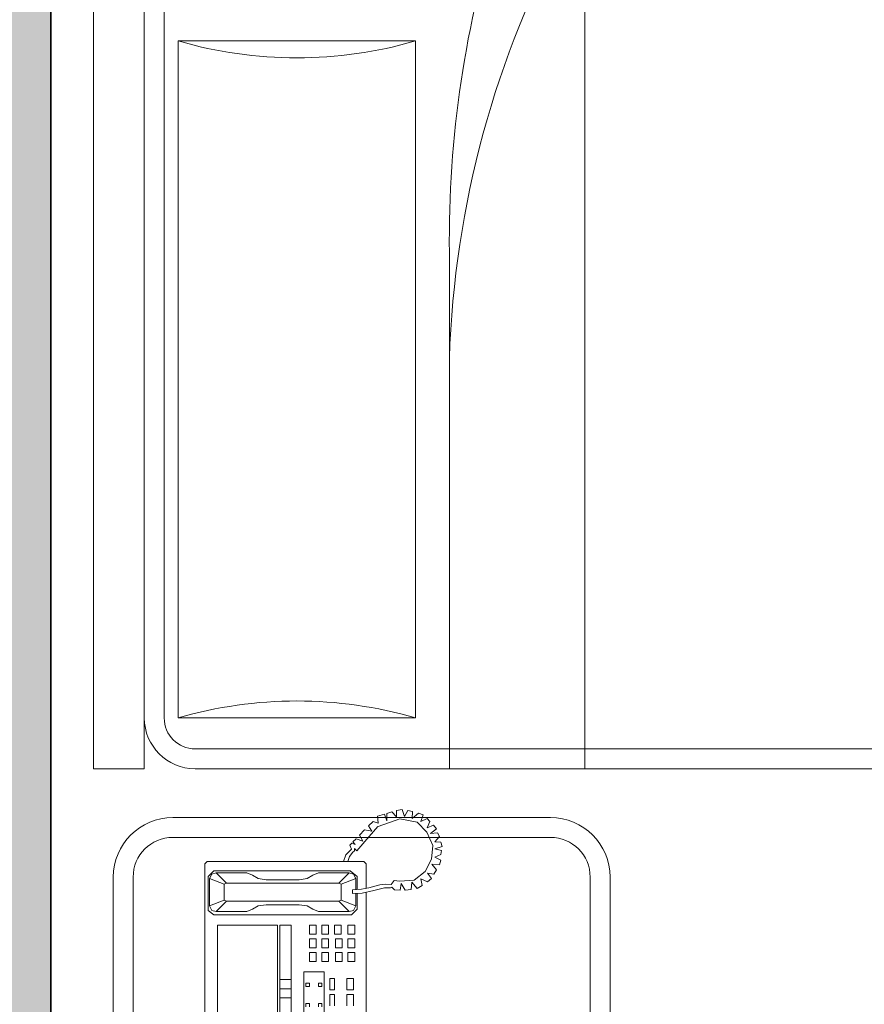
# Model space of a CAD drawing. Units: inches. Extents: x 2701 to 6846, y 811 to 2447.
# Tile 17 of 20: x 2977 to 3008, y 1370 to 1407. Entities that reach past the tile are written whole.
import ezdxf

# ---------------------------------------------------------------- set-up
doc = ezdxf.new("R2010")
doc.units = ezdxf.units.IN
for name, color, linetype, lineweight in [('A-FLOR-PATT', 252, 'Continuous', 13), ('A-FURN', 8, 'Continuous', 13), ('A-WALL', 7, 'Continuous', 35)]:
    doc.layers.add(name, color=color, linetype=linetype, lineweight=lineweight)
doc.layers.add('A-WALL-PATT', color=18, linetype='Continuous', lineweight=13, true_color=0x000000)

# ---------------------------------------------------------------- blocks, each defined once
blk = doc.blocks.new('A$C356F0359')
for p, q in [((0.5488961549126543, 2.000037877005524), (2.049197857799299, 2.000037877005524)), ((0.5488961549126543, 1.948857180890627), (0.5488961549126543, 2.000037877005524)), ((0.4397736946484656, 1.980067907948978), (0.059773694651085, 1.980067907948978)), ((0.4397736946484656, 1.960067907952179), (0.059773694651085, 1.960067907952179)), ((2.049197857799299, 1.948857180890627), (0.5488961549126543, 1.948857180890627)), ((1.998017161684401, 1.928857180893828), (0.6000768510275521, 1.928857180893828)), ((0.4797736946493388, 1.540067907953925), (0.4797736946493388, 1.920067907951306)), ((0.4997736946534133, 1.540067907953925), (0.4997736946534133, 1.920067907951306)), ((0.5488961549126543, 1.897676484783005), (0.5488961549126543, 0.0512185731204227)), ((0.5688961549167288, 1.897676484783005), (0.5688961549167288, 0.0512185731204227)), ((0.2724584284442244, 1.887891571575892), (0.4530524284491549, 1.887891571575892)), ((0.4016174284479348, 1.878747571572603), (0.4061894284459413, 1.88446257157193)), ((0.4061894284459413, 1.88446257157193), (0.44047942844918, 1.88446257157193)), ((0.44047942844918, 1.88446257157193), (0.4461944284485071, 1.878747571572603)), ((0.4530524284491549, 1.887891571575892), (0.4553384284445201, 1.88560557157325)), ((0.4553384284445201, 1.88560557157325), (0.4553384284445201, 1.727871571572904)), ((0.3913304284506012, 1.875318571575917), (0.2770304284495069, 1.875318571575917)), ((0.3913304284506012, 1.814739571571408), (0.3913304284506012, 1.875318571575917)), ((0.4016174284479348, 1.740444571572879), (0.4016174284479348, 1.878747571572603)), ((0.4061894284459413, 1.881033571575244), (0.4050464284446207, 1.876461571577237)), ((0.4050464284446207, 1.876461571577237), (0.4153334284492303, 1.866174571572628)), ((0.4050464284446207, 1.876461571577237), (0.4050464284446207, 1.845600571570685)), ((0.4107614284439478, 1.883319571570609), (0.4061894284459413, 1.881033571575244)), ((0.4107614284439478, 1.883319571570609), (0.4381934284465388, 1.883319571570609)), ((0.4164764284505509, 1.868460571575269), (0.4107614284439478, 1.883319571570609)), ((0.4324784284472117, 1.868460571575269), (0.4381934284465388, 1.883319571570609)), ((0.4439084284458659, 1.876461571577237), (0.4336214284485323, 1.866174571572628)), ((0.4381934284465388, 1.883319571570609), (0.4427654284445453, 1.881033571575244)), ((0.4427654284445453, 1.881033571575244), (0.4439084284458659, 1.876461571577237)), ((0.4439084284458659, 1.876461571577237), (0.4439084284458659, 1.845600571570685)), ((0.4461944284485071, 1.878747571572603), (0.4461944284485071, 1.7415875715742)), ((0.4153334284492303, 1.866174571572628), (0.4164764284505509, 1.868460571575269)), ((0.4153334284492303, 1.814739571571408), (0.4153334284492303, 1.866174571572628)), ((0.4324784284472117, 1.868460571575269), (0.4164764284505509, 1.868460571575269)), ((0.4336214284485323, 1.866174571572628), (0.4324784284472117, 1.868460571575269)), ((0.4336214284485323, 1.814739571571408), (0.4336214284485323, 1.866174571572628)), ((0.4050464284446207, 1.845600571570685), (0.407332428447262, 1.839885571571358)), ((0.4439084284458659, 1.845600571570685), (0.4416224284505006, 1.839885571571358)), ((0.407332428447262, 1.839885571571358), (0.4107614284439478, 1.83417057157203)), ((0.4416224284505006, 1.839885571571358), (0.4381934284465388, 1.83417057157203)), ((0.4107614284439478, 1.83417057157203), (0.4119044284452685, 1.826169571577338)), ((0.4119044284452685, 1.826169571577338), (0.4119044284452685, 1.814739571571408)), ((0.4381934284465388, 1.83417057157203), (0.4370504284452182, 1.826169571577338)), ((0.4370504284452182, 1.826169571577338), (0.4370504284452182, 1.814739571571408)), ((0.2770304284495069, 1.814739571571408), (0.3913304284506012, 1.814739571571408)), ((0.3913304284506012, 1.812453571576043), (0.2816024284475134, 1.812453571576043)), ((0.3181784284461173, 1.812453571576043), (0.3181784284461173, 1.801023571577388)), ((0.3273224284494063, 1.812453571576043), (0.3273224284494063, 1.801023571577388)), ((0.3364664284454193, 1.812453571576043), (0.3364664284454193, 1.801023571577388)), ((0.3913304284506012, 1.801023571577388), (0.3913304284506012, 1.812453571576043)), ((0.4119044284452685, 1.79302257157542), (0.4119044284452685, 1.814739571571408)), ((0.4153334284492303, 1.814739571571408), (0.4153334284492303, 1.753017571572854)), ((0.4336214284485323, 1.814739571571408), (0.4336214284485323, 1.753017571572854)), ((0.4370504284452182, 1.79302257157542), (0.4370504284452182, 1.814739571571408)), ((0.2816024284475134, 1.801023571577388), (0.3913304284506012, 1.801023571577388)), ((0.3444674284473876, 1.788450571577413), (0.2770304284495069, 1.788450571577413)), ((0.3124634284467902, 1.786164571574772), (0.3090344284501043, 1.786164571574772)), ((0.3124634284467902, 1.78273557157081), (0.3124634284467902, 1.786164571574772)), ((0.3330374284487334, 1.786164571574772), (0.3296084284447716, 1.786164571574772)), ((0.3296084284447716, 1.786164571574772), (0.3296084284447716, 1.78273557157081)), ((0.3330374284487334, 1.78273557157081), (0.3330374284487334, 1.786164571574772)), ((0.3444674284473876, 1.76787657157547), (0.3444674284473876, 1.788450571577413)), ((0.4107614284439478, 1.785021571573452), (0.4119044284452685, 1.79302257157542)), ((0.4381934284465388, 1.785021571573452), (0.4370504284452182, 1.79302257157542)), ((0.3090344284501043, 1.78273557157081), (0.3124634284467902, 1.78273557157081)), ((0.3296084284447716, 1.78273557157081), (0.3330374284487334, 1.78273557157081)), ((0.3547544284447213, 1.775877571577439), (0.3547544284447213, 1.78273557157081)), ((0.3547544284447213, 1.78273557157081), (0.3638984284480102, 1.78273557157081)), ((0.3638984284480102, 1.775877571577439), (0.3547544284447213, 1.775877571577439)), ((0.3638984284480102, 1.78273557157081), (0.3638984284480102, 1.775877571577439)), ((0.3684704284460167, 1.78273557157081), (0.3776144284493057, 1.78273557157081)), ((0.3684704284460167, 1.775877571577439), (0.3684704284460167, 1.78273557157081)), ((0.3776144284493057, 1.775877571577439), (0.3684704284460167, 1.775877571577439)), ((0.3776144284493057, 1.78273557157081), (0.3776144284493057, 1.775877571577439)), ((0.3821864284473122, 1.775877571577439), (0.3821864284473122, 1.78273557157081)), ((0.3821864284473122, 1.78273557157081), (0.3913304284506012, 1.78273557157081)), ((0.3913304284506012, 1.775877571577439), (0.3821864284473122, 1.775877571577439)), ((0.3913304284506012, 1.78273557157081), (0.3913304284506012, 1.775877571577439)), ((0.4050464284446207, 1.773591571574797), (0.407332428447262, 1.779306571574124)), ((0.407332428447262, 1.779306571574124), (0.4107614284439478, 1.785021571573452)), ((0.4416224284505006, 1.779306571574124), (0.4381934284465388, 1.785021571573452)), ((0.4439084284458659, 1.773591571574797), (0.4416224284505006, 1.779306571574124)), ((0.2770304284495069, 1.76787657157547), (0.3444674284473876, 1.76787657157547)), ((0.3124634284467902, 1.773591571574797), (0.3090344284501043, 1.773591571574797)), ((0.3090344284501043, 1.770162571570836), (0.3124634284467902, 1.770162571570836)), ((0.3124634284467902, 1.770162571570836), (0.3124634284467902, 1.773591571574797)), ((0.3330374284487334, 1.773591571574797), (0.3296084284447716, 1.773591571574797)), ((0.3296084284447716, 1.773591571574797), (0.3296084284447716, 1.770162571570836)), ((0.3296084284447716, 1.770162571570836), (0.3330374284487334, 1.770162571570836)), ((0.3330374284487334, 1.770162571570836), (0.3330374284487334, 1.773591571574797)), ((0.3547544284447213, 1.763304571577464), (0.3547544284447213, 1.770162571570836)), ((0.3547544284447213, 1.770162571570836), (0.3638984284480102, 1.770162571570836)), ((0.3638984284480102, 1.770162571570836), (0.3638984284480102, 1.763304571577464)), ((0.3684704284460167, 1.763304571577464), (0.3684704284460167, 1.770162571570836)), ((0.3684704284460167, 1.770162571570836), (0.3776144284493057, 1.770162571570836)), ((0.3776144284493057, 1.770162571570836), (0.3776144284493057, 1.763304571577464)), ((0.3821864284473122, 1.763304571577464), (0.3821864284473122, 1.770162571570836)), ((0.3821864284473122, 1.770162571570836), (0.3913304284506012, 1.770162571570836)), ((0.3913304284506012, 1.770162571570836), (0.3913304284506012, 1.763304571577464)), ((0.4050464284446207, 1.742730571575521), (0.4050464284446207, 1.773591571574797)), ((0.4439084284458659, 1.742730571575521), (0.4439084284458659, 1.773591571574797)), ((0.3216074284500792, 1.762161571576143), (0.310177428444149, 1.762161571576143)), ((0.310177428444149, 1.757589571570861), (0.3216074284500792, 1.757589571570861)), ((0.3216074284500792, 1.757589571570861), (0.3216074284500792, 1.762161571576143)), ((0.3376094284467399, 1.762161571576143), (0.3261794284480857, 1.762161571576143)), ((0.3261794284480857, 1.762161571576143), (0.3261794284480857, 1.757589571570861)), ((0.3261794284480857, 1.757589571570861), (0.3376094284467399, 1.757589571570861)), ((0.3376094284467399, 1.757589571570861), (0.3376094284467399, 1.762161571576143)), ((0.3638984284480102, 1.763304571577464), (0.3547544284447213, 1.763304571577464)), ((0.3547544284447213, 1.756446571576816), (0.3638984284480102, 1.756446571576816)), ((0.3547544284447213, 1.749588571576168), (0.3547544284447213, 1.756446571576816)), ((0.3638984284480102, 1.756446571576816), (0.3638984284480102, 1.749588571576168)), ((0.3776144284493057, 1.763304571577464), (0.3684704284460167, 1.763304571577464)), ((0.3684704284460167, 1.756446571576816), (0.3776144284493057, 1.756446571576816)), ((0.3684704284460167, 1.749588571576168), (0.3684704284460167, 1.756446571576816)), ((0.3776144284493057, 1.756446571576816), (0.3776144284493057, 1.749588571576168)), ((0.3913304284506012, 1.763304571577464), (0.3821864284473122, 1.763304571577464)), ((0.3821864284473122, 1.757589571570861), (0.3913304284506012, 1.757589571570861)), ((0.3821864284473122, 1.750731571577489), (0.3821864284473122, 1.757589571570861)), ((0.3913304284506012, 1.757589571570861), (0.3913304284506012, 1.750731571577489)), ((0.3638984284480102, 1.749588571576168), (0.3547544284447213, 1.749588571576168)), ((0.3776144284493057, 1.749588571576168), (0.3684704284460167, 1.749588571576168)), ((0.3913304284506012, 1.750731571577489), (0.3821864284473122, 1.750731571577489)), ((0.4050464284446207, 1.742730571575521), (0.4153334284492303, 1.753017571572854)), ((0.4164764284505509, 1.750731571577489), (0.4107614284439478, 1.735872571574873)), ((0.4153334284492303, 1.753017571572854), (0.4164764284505509, 1.750731571577489)), ((0.4324784284472117, 1.750731571577489), (0.4164764284505509, 1.750731571577489)), ((0.4336214284485323, 1.753017571572854), (0.4324784284472117, 1.750731571577489)), ((0.4324784284472117, 1.750731571577489), (0.4381934284465388, 1.735872571574873)), ((0.4439084284458659, 1.742730571575521), (0.4336214284485323, 1.753017571572854)), ((0.4621985062476597, 1.745894538602442), (0.4553384284445201, 1.748445571574848)), ((0.4654197563650087, 1.742671277948829), (0.4621985062476597, 1.745894538602442)), ((0.310177428444149, 1.745016571570886), (0.3216074284500792, 1.745016571570886)), ((0.3216074284500792, 1.738158571577514), (0.310177428444149, 1.738158571577514)), ((0.3216074284500792, 1.745016571570886), (0.3216074284500792, 1.738158571577514)), ((0.3261794284480857, 1.738158571577514), (0.3261794284480857, 1.745016571570886)), ((0.3261794284480857, 1.745016571570886), (0.3376094284467399, 1.745016571570886)), ((0.3376094284467399, 1.738158571577514), (0.3261794284480857, 1.738158571577514)), ((0.3376094284467399, 1.745016571570886), (0.3376094284467399, 1.738158571577514)), ((0.3547544284447213, 1.737015571576193), (0.3547544284447213, 1.743873571576841)), ((0.3547544284447213, 1.743873571576841), (0.3638984284480102, 1.743873571576841)), ((0.3638984284480102, 1.737015571576193), (0.3547544284447213, 1.737015571576193)), ((0.3638984284480102, 1.743873571576841), (0.3638984284480102, 1.737015571576193)), ((0.3684704284460167, 1.737015571576193), (0.3684704284460167, 1.743873571576841)), ((0.3684704284460167, 1.743873571576841), (0.3776144284493057, 1.743873571576841)), ((0.3776144284493057, 1.737015571576193), (0.3684704284460167, 1.737015571576193)), ((0.3776144284493057, 1.743873571576841), (0.3776144284493057, 1.737015571576193)), ((0.3821864284473122, 1.743873571576841), (0.3913304284506012, 1.743873571576841)), ((0.3821864284473122, 1.737015571576193), (0.3821864284473122, 1.743873571576841)), ((0.3913304284506012, 1.737015571576193), (0.3821864284473122, 1.737015571576193)), ((0.3913304284506012, 1.743873571576841), (0.3913304284506012, 1.737015571576193)), ((0.407332428447262, 1.734729571573552), (0.4016174284479348, 1.740444571572879)), ((0.4061894284459413, 1.738158571577514), (0.4050464284446207, 1.742730571575521)), ((0.4107614284439478, 1.735872571574873), (0.4061894284459413, 1.738158571577514)), ((0.4107614284439478, 1.735872571574873), (0.4233900228064158, 1.735872571574873)), ((0.4233344284439227, 1.739301571571559), (0.423494239061256, 1.729444625765609)), ((0.4267634284478845, 1.739301571571559), (0.4233344284439227, 1.739301571571559)), ((0.4274265633430332, 1.730138997823814), (0.4267634284478845, 1.739301571571559)), ((0.4270115999388509, 1.735872571574873), (0.4381934284465388, 1.735872571574873)), ((0.4381934284465388, 1.735872571574873), (0.4427654284445453, 1.738158571577514)), ((0.4461944284485071, 1.7415875715742), (0.44047942844918, 1.734729571573552)), ((0.4427654284445453, 1.738158571577514), (0.4439084284458659, 1.742730571575521)), ((0.4553384284445201, 1.743873571576841), (0.460386552316777, 1.742469824450381)), ((0.460386552316777, 1.742469824450381), (0.465017100199475, 1.738843656814424)), ((0.465017100199475, 1.738843656814424), (0.4662250694818795, 1.73723202648398)), ((0.4678356941440143, 1.740455287137592), (0.4654197563650087, 1.742671277948829)), ((0.4662250694818795, 1.73723202648398), (0.4686410072681611, 1.737433481161133)), ((0.4686410072681611, 1.737433481161133), (0.4662250694818795, 1.735016035672742)), ((0.4720635858611786, 1.742066917460761), (0.4678356941440143, 1.740455287137592)), ((0.4740768674819265, 1.740052378961991), (0.4720635858611786, 1.742066917460761)), ((0.4724662420267123, 1.736627666003187), (0.4740768674819265, 1.740052378961991)), ((0.4752848359785276, 1.738843656814424), (0.4724662420267123, 1.736627666003187)), ((0.4783047584060114, 1.735620397346792), (0.4752848359785276, 1.738843656814424)), ((0.4234085542557296, 1.734729571573552), (0.407332428447262, 1.734729571573552)), ((0.423494239061256, 1.729444625765609), (0.4262699974206044, 1.717871750719496)), ((0.44047942844918, 1.734729571573552), (0.4270943237643224, 1.734729571573552)), ((0.4290457557799528, 1.722732358299253), (0.4274265633430332, 1.730138997823814)), ((0.4553384284445201, 1.727871571572904), (0.4530524284491549, 1.725585571577539)), ((0.4662250694818795, 1.735016035672742), (0.4754861644541962, 1.726756431737157)), ((0.4754861644541962, 1.726756431737157), (0.4905857757985359, 1.713863391494669)), ((0.4758888206197299, 1.728972422541119), (0.4783047584060114, 1.735620397346792)), ((0.4821299939503661, 1.732195683194731), (0.4758888206197299, 1.728972422541119)), ((0.4873645256884629, 1.727159339905483), (0.4821299939503661, 1.732195683194731)), ((0.4861565563987825, 1.719907004626293), (0.4873645256884629, 1.727159339905483)), ((0.4244198346350459, 1.725585571577539), (0.2724584284442244, 1.725585571577539)), ((0.4262699974206044, 1.717871750719496), (0.4290457557799528, 1.706993247731588)), ((0.4530524284491549, 1.725585571577539), (0.4284220044355607, 1.725585571577539)), ((0.4318215141393012, 1.711853855318622), (0.4290457557799528, 1.722732358299253)), ((0.4913910889226827, 1.723130264093924), (0.4861565563987825, 1.719907004626293)), ((0.4958203083224362, 1.718496827794297), (0.4913910889226827, 1.723130264093924)), ((0.4940083551846329, 1.713460484505048), (0.4958203083224362, 1.718496827794297)), ((0.4290457557799528, 1.706993247731588), (0.4288144428792294, 1.700975353385729)), ((0.4325154535545153, 1.706298875673383), (0.4318215141393012, 1.711853855318622)), ((0.4322841406537919, 1.700280980272509), (0.4325154535545153, 1.706298875673383)), ((0.4908063805487473, 1.713474057840358), (0.4984397162188543, 1.691717052926833)), ((0.5009841616774793, 1.714168430953577), (0.4940447654225864, 1.713474057840358)), ((0.4963578972747201, 1.704678673144371), (0.5030659799231217, 1.707224706136912)), ((0.5030659799231217, 1.707224706136912), (0.5009841616774793, 1.714168430953577)), ((0.4269639368358185, 1.697040575214487), (0.4265013103213278, 1.691485595576523)), ((0.4295083822944435, 1.699586608207027), (0.4269639368358185, 1.697040575214487)), ((0.4288144428792294, 1.700975353385729), (0.4295083822944435, 1.699586608207027)), ((0.4364477785493364, 1.69727203361981), (0.4322841406537919, 1.700280980272509)), ((0.435522525527631, 1.691948510277143), (0.4364477785493364, 1.69727203361981)), ((0.5037599200368277, 1.704910130501957), (0.4963578972747201, 1.704678673144371)), ((0.5005215351702647, 1.694957457984855), (0.5053791124737473, 1.699586608207027)), ((0.5053791124737473, 1.699586608207027), (0.5037599200368277, 1.704910130501957)), ((0.4265013103213278, 1.691485595576523), (0.4332093936754973, 1.690328307755407)), ((0.4332093936754973, 1.690328307755407), (0.4267326239278191, 1.686393530639179)), ((0.4267326239278191, 1.686393530639179), (0.4271952504423098, 1.68014417788072)), ((0.4366790914500598, 1.677366687537869), (0.435522525527631, 1.691948510277143)), ((0.4984397162188543, 1.691717052926833), (0.4952013313522912, 1.67435774088517)), ((0.5067669913041755, 1.694957457984855), (0.5005215351702647, 1.694957457984855)), ((0.500752848070988, 1.687087902697385), (0.5079235572338803, 1.68917102098203)), ((0.5067669913041755, 1.683616040289052), (0.500752848070988, 1.687087902697385)), ((0.5079235572338803, 1.68917102098203), (0.5067669913041755, 1.694957457984855)), ((0.4271952504423098, 1.68014417788072), (0.4345972725059255, 1.679449805822514)), ((0.4345972725059255, 1.679449805822514), (0.4281205027582474, 1.67435774088517)), ((0.4454689930425957, 1.66625672824739), (0.4366790914500598, 1.677366687537869)), ((0.5042225465513184, 1.672968995713745), (0.4986710291268537, 1.679218348464928)), ((0.4986710291268537, 1.679218348464928), (0.5058417382824701, 1.678986890059604)), ((0.5058417382824701, 1.678986890059604), (0.5067669913041755, 1.683616040289052)), ((0.4281205027582474, 1.67435774088517), (0.431127574731363, 1.669034217542503)), ((0.431127574731363, 1.669034217542503), (0.4380669702804881, 1.670422962721204)), ((0.4380669702804881, 1.670422962721204), (0.4348285861124169, 1.663942152605159)), ((0.4577285924169701, 1.65977591813862), (0.4454689930425957, 1.66625672824739)), ((0.4952013313522912, 1.67435774088517), (0.4850235502235592, 1.664405068368068)), ((0.4956639578595059, 1.670422962721204), (0.5023720405079076, 1.668339845484297)), ((0.498902342733345, 1.664173609962745), (0.4956639578595059, 1.670422962721204)), ((0.5023720405079076, 1.668339845484297), (0.5042225465513184, 1.672968995713745)), ((0.4348285861124169, 1.663942152605159), (0.4382982838869794, 1.65977591813862)), ((0.4382982838869794, 1.65977591813862), (0.4436184877049528, 1.663710695254849)), ((0.4436184877049528, 1.663710695254849), (0.4426932346832473, 1.657461342496389)), ((0.4426932346832473, 1.657461342496389), (0.4470881854795153, 1.654683853201277)), ((0.4470881854795153, 1.654683853201277), (0.452639702205488, 1.659313003430725)), ((0.452639702205488, 1.659313003430725), (0.4519457627902739, 1.65167490550084)), ((0.4568033401010326, 1.650286160329414), (0.4598104113611044, 1.656535513087874)), ((0.471607384926756, 1.658618630317505), (0.4577285924169701, 1.65977591813862)), ((0.4598104113611044, 1.656535513087874), (0.4625861697277287, 1.650286160329414)), ((0.4665184947152739, 1.649823245621519), (0.4681376864464255, 1.656535513087874)), ((0.4681376864464255, 1.656535513087874), (0.4706821319050505, 1.649128872508299)), ((0.4850235502235592, 1.664405068368068), (0.471607384926756, 1.658618630317505)), ((0.4750770827013185, 1.650286160329414), (0.4753083963078098, 1.656535513087874)), ((0.4753083963078098, 1.656535513087874), (0.4806285994272912, 1.651906362858426)), ((0.4843296108083451, 1.653758022737747), (0.4836356713931309, 1.660701747554412)), ((0.4836356713931309, 1.660701747554412), (0.4884932487038896, 1.654683853201277)), ((0.4884932487038896, 1.654683853201277), (0.4921942600849434, 1.657924258259299)), ((0.4921942600849434, 1.657924258259299), (0.4894185010198271, 1.664173609962745)), ((0.4894185010198271, 1.664173609962745), (0.4958952707602294, 1.661396120667632)), ((0.4958952707602294, 1.661396120667632), (0.498902342733345, 1.664173609962745)), ((0.4519457627902739, 1.65167490550084), (0.4568033401010326, 1.650286160329414)), ((0.4625861697277287, 1.650286160329414), (0.4665184947152739, 1.649823245621519)), ((0.4706821319050505, 1.649128872508299), (0.4750770827013185, 1.650286160329414)), ((0.4806285994272912, 1.651906362858426), (0.4843296108083451, 1.653758022737747)), ((0.059773694651085, 1.500067907953052), (0.4397736946484656, 1.500067907953052)), ((0.059773694651085, 1.480067907948978), (0.4397736946484656, 1.480067907948978))]:
    blk.add_line(p, q)
at = {"linetype": 'ByBlock'}
for p, q in [((0.6000768510275521, 1.914736716818879), (1.281986774316465, 1.914736716818879)), ((0.6000768510275521, 1.675893468294816), (0.6000768510275521, 1.914736716818879)), ((1.281986774316465, 1.914736716818879), (1.281986774316465, 1.675893468294816)), ((1.281986774316465, 1.675893468294816), (0.6000768510275521, 1.675893468294816)), ((1.068733873849851, 1.641773004215792), (0.5488961549126543, 1.641773004215792)), ((1.418468630618008, 1.505291147914249), (0.5488961549126543, 1.505291147914249))]:
    blk.add_line(p, q, dxfattribs=at)
for centre, radius, start, end in [((0.4397736946484656, 1.920067907951306), 0.06, 0, 90), ((0.4397736946484656, 1.920067907951306), 0.0399999999999855, 0, 90), ((0.6000768510275521, 1.897676484783005), 0.0511806961126753, 90, 180), ((0.6000768510275521, 1.897676484783005), 0.0311806961126753, 90, 180), ((0.4397736946484656, 1.540067907953925), 0.04, 270, 0), ((0.4397736946484656, 1.540067907953925), 0.06, 270, 0)]:
    blk.add_arc(centre, radius, start, end)
for centre, radius, start, end in [((0.1906312821229221, 1.795315092553209), 0.4265058009389605, 343.7397948414725, 16.26020515852748), ((1.691432343221094, 1.795315092553209), 0.4265058009389605, 163.7397948414725, 196.2602051585274), ((0.9302674239734187, 0.6570376961535658), 0.9852622038361044, 61.43284801268289, 88.12613015168571), ((1.082595312378543, 0.5712434438610217), 1.070619297177308, 72.19663287785316, 90.74183579771547)]:
    blk.add_arc(centre, radius, start, end, dxfattribs=at)

msp = doc.modelspace()

# ---------------------------------------------------------------- hatches: boundary and pattern name
at = {"layer": 'A-FLOR-PATT'}
h = msp.add_hatch(dxfattribs=at)
h.set_pattern_fill('ANGLE', color=256)
h.set_pattern_definition([(0, (0, 0), (0, 6.985), [5.08, -1.905]), (90, (0, 0), (-6.985, 4e-16), [5.08, -1.905])])
h.paths.add_polyline_path([(2841.812531618507, 1296.510714093028, -0.1094531397224823), (2842.614165366529, 1300.128842847245, -0.1023747835315324), (2844.977063233859, 1303.301704019213, -0.0937428406070795), (2848.425874088265, 1305.367635711971, -0.0624630522953803), (2851.366818664733, 1306.050044742079), (2785.971391037217, 1306.050044742079), (2785.971391037217, 1258.050044742079), (2827.971391037217, 1258.050044742079), (2827.971391037217, 1256.411537864998), (2829.450762355621, 1256.411537864998, -0.3948265708167148), (2854.747422469505, 1283.452795228435), (2856.49201971855, 1283.452795228435), (2856.49201971876, 1256.411537865324), (2857.971391037219, 1256.411537865324), (2857.971391037219, 1258.05004474208), (2863.971391037218, 1258.050044742079), (2863.971391037217, 1306.050044742079), (2853.867060923166, 1306.050044742079, -0.0624630504647152), (2856.808005416599, 1305.367635742541, -0.0937428427235612), (2860.256816355725, 1303.301704017657, -0.1023747714125829), (2862.619714024758, 1300.128843269809, -0.1094531521575188), (2863.421347969692, 1296.510714138194, -0.109453153989093), (2862.619714017641, 1292.892584946142, -0.1023747709767553), (2860.256816355757, 1289.719724213534, -0.093738257087872), (2856.808189965141, 1287.653860434733, -0.0884250558281599), (2852.616939784454, 1286.906795737127, -0.0884250554332989), (2848.425689622791, 1287.653860434813, -0.0937382570330623), (2844.977063234018, 1289.719724212192, -0.1023747824199799), (2842.614165384649, 1292.892585345091, -0.1094531396555831)])
h.paths.add_polyline_path([(2805.214857085719, 1273.877134568363, -0.141745245190178), (2808.318689175414, 1271.772621468736, -0.1849834247598648), (2809.773740825251, 1267.974277286972, -0.1849834247688995), (2808.318689175285, 1264.175933105053, -0.141745244968364), (2805.214857091107, 1262.071420007333, -0.1522440861962393), (2799.994488829542, 1261.79557176336, -0.0256138964539793), (2799.368711507224, 1261.94541476925), (2794.365115778627, 1263.418098821323), (2794.36467071784, 1263.405353947873, -0.1112416791490392), (2793.99312620013, 1261.915170284834, -0.0338893268367682), (2793.114424873909, 1260.113565580275, -0.286745385218), (2792.375651823606, 1259.651928944151), (2787.580775843661, 1259.651928944133, -0.4142135623681101), (2787.152671505053, 1260.080033282747), (2787.152671505153, 1267.974277286972), (2787.152671505053, 1275.868521290948, -0.4142135623730951), (2787.580775843668, 1276.296625629562), (2792.375651823623, 1276.296625629544, -0.2867453846084762), (2793.114424873105, 1275.834988995069, -0.0338893268640583), (2793.99312620013, 1274.033384289111, -0.1051042356073151), (2794.361711671137, 1272.627936636842), (2794.365115778619, 1272.530455752619), (2799.368711507498, 1274.003139804786, -0.0256138965941945), (2799.994488833287, 1274.152982811292, -0.1522440859162748)], flags=16)
h.paths.add_polyline_path([(2804.681063364808, 1272.339952816459, -0.1449445299175104), (2807.087654609562, 1270.708506585421, -0.0358001151589041), (2807.447023191777, 1270.252713401882, -0.1332846890906797), (2807.893417732773, 1268.607871708063), (2807.893417732813, 1267.974277286972), (2807.893417732773, 1267.340682865632, -0.1332846888970446), (2807.447023193029, 1265.695841173949, -0.0358001152638917), (2807.087654609923, 1265.240047988954, -0.1449445297267833), (2804.681063368992, 1263.608601758809, -0.1554037438169349), (2800.343099481134, 1263.385728797012, -0.3645106918446579), (2796.485382154562, 1267.974277286972, -0.3645106920174053), (2800.343099483932, 1272.562825777418, -0.1554037435534987)], flags=0)
h.paths.add_polyline_path([(2800.015880108981, 1268.901471623875, 0.1692977046764319), (2799.131174998024, 1268.11576383613, 0.0766670309700064), (2799.100009657075, 1267.974277286936, 0.0766670313951798), (2799.13117499834, 1267.832790736999, 0.1692977045836763), (2800.015880108981, 1267.04708294982, 0.3052192884941762), (2800.365297210358, 1267.156497374013, 0.1695347489604994), (2800.650786991011, 1267.974277286972, 0.1695347391656343), (2800.365297241503, 1268.792057160761, 0.3052193300480048)], flags=0)
h.paths.add_polyline_path([(2971.971391037218, 1456.050044742079), (2923.971391037218, 1456.050044742079), (2923.971391037218, 1408.050044742079), (2922.332884160136, 1408.050044742079), (2922.332884160136, 1406.570673423676, -0.394826570816717), (2949.374141523573, 1381.274013309792), (2949.374141523573, 1379.529416060747), (2922.332884160461, 1379.529416060537), (2922.332884160461, 1378.050044742079), (2923.971391037218, 1378.050044742079), (2923.971391037217, 1372.050044742079), (2971.971391037217, 1372.050044742079)])
h.paths.add_polyline_path([(2939.8177624336, 1436.526417411941, -0.1417452451905352), (2937.713249333971, 1433.422585322236, -0.1849834247599418), (2933.914905152205, 1431.967533672398, -0.1849834247691276), (2930.116560970283, 1433.422585322367, -0.1417452449676952), (2928.01204787257, 1436.526417406529, -0.1522440861964963), (2927.736199628592, 1441.746785668103, -0.0256138964540868), (2927.886042634483, 1442.372562990423), (2929.358726686557, 1447.376158719022), (2929.345981813088, 1447.376603779809, -0.1112416791473441), (2927.855798150072, 1447.748148297517, -0.0338893268369074), (2926.054193445506, 1448.626849623741, -0.2867453852169366), (2925.592556809384, 1449.365622674043), (2925.592556809366, 1454.160498653989, -0.4142135623681173), (2926.020661147981, 1454.588602992596), (2933.914905152205, 1454.588602992496), (2941.809149156182, 1454.588602992596, -0.4142072303161659), (2942.237253494696, 1454.160507909187), (2942.237253494777, 1449.365622674043, -0.2867453846243844), (2941.775616860276, 1448.626849624529, -0.0338893268635044), (2939.974012154347, 1447.74814829752, -0.1051042356087532), (2938.568564502058, 1447.379562826511), (2938.471083617852, 1447.37615871903), (2939.943767670019, 1442.372562990154, -0.0256138965942444), (2940.093610676525, 1441.746785664364, -0.152244085915992)], flags=16)
h.paths.add_polyline_path([(2938.280580681695, 1437.060211132847, -0.1449445299182329), (2936.649134450649, 1434.653619888082, -0.0358001151583613), (2936.193341267117, 1434.294251305872, -0.1332846890907526), (2934.548499573297, 1433.847856764876), (2933.914905152205, 1433.847856764836), (2933.281310730865, 1433.847856764876, -0.1332846888976268), (2931.636469039176, 1434.294251304624, -0.0358001152630847), (2931.180675854191, 1434.653619887722, -0.14494452972667), (2929.549229624045, 1437.06021112865, -0.1554037438170702), (2929.326356662246, 1441.398175016512, -0.3645106918448713), (2933.914905152205, 1445.255892343087, -0.3645106920173691), (2938.503453642651, 1441.398175013717, -0.1554037435532691)], flags=0)
h.paths.add_polyline_path([(2969.158462562638, 1392.044508285666, -0.0937428443921736), (2971.224394311477, 1388.595697278927, -0.0884209696484748), (2971.971391037217, 1384.404631716083, -0.0884209680179829), (2971.224394332037, 1380.213566228077, -0.0937428458331012), (2969.158462561081, 1376.764755163806, -0.1023747798731684), (2965.985601516888, 1374.401857356678, -0.1094531425013952), (2962.367472681615, 1373.600223549837, -0.1094531553411192), (2958.74934344807, 1374.401857521223, -0.102374769792102), (2955.576482756955, 1376.764755163771, -0.0937382570879047), (2953.510618978154, 1380.213381554388, -0.0884250558281564), (2952.763554280548, 1384.404631735075, -0.0884250554336261), (2953.510618978239, 1388.595881896752, -0.0937382570324601), (2955.576482755607, 1392.044508285504, -0.1023747638736991), (2958.749343238892, 1394.40740583216, -0.10945316082308), (2962.367472636449, 1395.209039901022, -0.1094531494878097), (2965.985601690358, 1394.407406013345, -0.102374774975509)], flags=0)
edge = h.paths.add_edge_path(flags=16)
edge.add_arc((2961.074722408913, 1384.858947505427), 10.19921062335061, 20.21320321302568, 41.63359467655653, ccw=False)
edge.add_spline(control_points=[(2970.645798607602, 1388.382922212802), (2970.45927694694, 1387.830081875375), (2970.004018351208, 1386.480719475378), (2971.435235818619, 1384.395639569603), (2969.86804662324, 1382.338798369057), (2970.408139739579, 1381.010733700175), (2970.645798607602, 1380.426341238356)], knot_values=[0, 0, 0, 0, 0.0411087303528805, 0.1003374234737184, 0.1559132068848227, 0.1995857666183122, 0.1995857666183122, 0.1995857666183122, 0.1995857666183122], degree=3, periodic=0)
edge.add_arc((2961.074722408954, 1383.950315945844), 10.19921062335061, 318.3664053106646, 339.7867967863075, ccw=False)
edge.add_arc((2961.862292702369, 1383.250252100635), 9.145476143303874, 294.98529005245234, 318.3664053112933, ccw=False)
edge.add_arc((2962.367474738348, 1382.166141072693), 7.949438681384353, 269.9999862429006, 294.9853451035073, ccw=False)
edge.add_arc((2962.367470579714, 1382.166141072693), 7.949438681384465, 245.0146528606722, 270.00001621636034, ccw=False)
edge.add_arc((2962.872652615592, 1383.250252100682), 9.145476143303885, 221.633594689284, 245.0147081786685, ccw=False)
edge.add_arc((2963.660222908995, 1383.950315945905), 10.19921062335051, 200.2129623510071, 221.6335946899624, ccw=False)
edge.add_arc((2964.894158186733, 1384.404632705954), 11.5141250647146, 180.0000045856949, 200.2129623497761, ccw=False)
edge.add_arc((2964.894158186734, 1384.404630744956), 11.51412506471477, 159.7870376490639, 179.999994827515, ccw=False)
edge.add_arc((2963.660222908922, 1384.858947504804), 10.19921062335051, 138.3664053200289, 159.7870376464858, ccw=False)
edge.add_arc((2962.872652615694, 1385.559011350224), 9.145476143303881, 114.9852895697228, 138.3664053235114, ccw=False)
edge.add_arc((2962.367470579715, 1386.643122378167), 7.949438681384341, 89.99998624290072, 114.9853445481478, ccw=False)
edge.add_arc((2962.367474738348, 1386.643122378167), 7.949438681384461, 65.01465414332972, 90.00001621635698, ccw=False)
edge.add_arc((2961.862292702924, 1385.559011349966), 9.145476143303876, 41.63359468007258, 65.01470929671348, ccw=False)
h.paths.add_polyline_path([(2963.809881193461, 1393.327235568244, -0.1264579126559968), (2966.613496696745, 1390.682864813822, -0.1416969839114421), (2967.169431848072, 1388.76054773013), (2967.169431848171, 1387.405856218539, -1), (2969.570411442753, 1387.40585621857, -0.4142135626407067), (2968.369921644365, 1386.205366421279), (2963.567962456663, 1385.004876624353, 0.146217798515541), (2963.311249278865, 1384.663463983469), (2968.97016654397, 1385.639690083447), (2968.97016654397, 1383.154510596366), (2963.317428127216, 1384.129674263443, 0.1403115373898127), (2963.56796245605, 1383.804386826958), (2968.369921645561, 1382.603897029581, -0.4142135623489124), (2969.570411442753, 1381.403407232289, -1), (2967.169431848171, 1381.403407232289), (2967.169431848072, 1380.040463554169, -0.1490250791000606), (2966.557068512987, 1378.031526062613, -0.0127594246128423), (2966.264512020975, 1377.619349736432, -0.1063032105074506), (2963.809880694587, 1375.482028786924, -0.1268223860120219), (2961.166982861567, 1374.800713347196, -0.12682239841106), (2958.52408452876, 1375.482027883284, -0.1063031789236789), (2956.069454414507, 1377.619348785205, -0.0857220920089208), (2954.537253221299, 1380.622635309784, -0.0753510219692474), (2953.964044077883, 1384.404631725429, -0.0753510220208753), (2954.537253222076, 1388.186628143578, -0.0857220919249397), (2956.069454414099, 1391.189914665108, -0.1063031717113424), (2958.5240850283, 1393.327234664099, -0.1268223860250843), (2961.166982861567, 1394.008550103962, -0.1268223983642548)], flags=0)
h.paths.add_polyline_path([(2934.842099489099, 1441.725394388693, 0.1692977046741335), (2934.056391701355, 1442.610099499628, 0.0766670309649834), (2933.91490515217, 1442.641264840574, 0.0766670314095982), (2933.773418602207, 1442.610099499295, 0.1692977045780331), (2932.987710815057, 1441.72539438868, 0.305219290057435), (2933.097125240708, 1441.375977286128, 0.169534748594888), (2933.914905152205, 1441.090487506638, 0.1695347390414705), (2934.732685025499, 1441.375977255749, 0.3052193305973386)], flags=0)
h.paths.add_polyline_path([(2969.323819906164, 1387.40585621857, -1), (2967.416023384759, 1387.40585621857, -1)], flags=0)
h.paths.add_polyline_path([(2968.830636832988, 1387.40585621857, -1), (2967.909206457936, 1387.40585621857, -1)], flags=0)
h.paths.add_polyline_path([(2962.129657139981, 1384.357435236314, -1), (2960.208873464314, 1384.357435236314, -1)], flags=0)
h.paths.add_polyline_path([(2961.800868424529, 1384.357435236314, -1), (2960.537662179766, 1384.357435236314, -1)], flags=0)
h.paths.add_polyline_path([(2969.323819906164, 1381.403407232289, -1), (2967.416023384759, 1381.403407232289, -1)], flags=0)
h.paths.add_polyline_path([(2968.830636832988, 1381.403407232289, -1), (2967.909206457936, 1381.403407232289, -1)], flags=0)
h.paths.add_polyline_path([(3085.971391037217, 1306.050044742079), (3001.971391037217, 1306.050044742079), (3001.971391037217, 1300.050044742079), (3000.332884160462, 1300.050044742079), (3000.332884160462, 1298.570673423621), (3027.374141523574, 1298.570673423411), (3027.374141523574, 1296.826076174374, -0.3948265708167921), (3000.332884160137, 1271.529416060482), (3000.332884160137, 1270.050044742079), (3001.971391037216, 1270.050044742079), (3001.971391037217, 1258.050044742079), (3085.971391037217, 1258.050044742079)])
h.paths.add_polyline_path([(3033.332715044416, 1274.444953022308, -0.1023747723857111), (3035.695612729331, 1271.272092240373, -0.1094531510467398), (3036.49724665838, 1267.653963142847, -0.109453129065687), (3035.695613062762, 1264.035834715682, -0.102374792813879), (3033.332715044451, 1260.862973218194, -0.0937428491083937), (3029.883903848349, 1258.797041398739, -0.0884209654955001), (3025.692838473141, 1258.05004474208, -0.0884209669723455), (3021.501773032378, 1258.797041429867, -0.093742846952782), (3018.052961922706, 1260.862973216846, -0.1023747779170817), (3015.690064146835, 1264.035834192024, -0.1094531447948728), (3014.888430307195, 1267.653963097683, -0.1094531229044609), (3015.690063814699, 1271.272091335764, -0.1023747982671114), (3018.052961922546, 1274.444953023867, -0.0937382570344717), (3021.501588311451, 1276.510816801145, -0.0884250558280669), (3025.692838492134, 1277.25788149875, -0.0884250554332868), (3029.884088653796, 1276.510816801064, -0.0937382570874262)], flags=0)
edge = h.paths.add_edge_path(flags=16)
edge.add_arc((3026.847218107582, 1267.148783163603), 9.145476143303444, 24.985288685417686, 48.36640531129461, ccw=False)
edge.add_arc((3027.931329135525, 1267.653965199581), 7.949438681383711, -1.3757099395661498e-05, 24.98534353079839, ccw=False)
edge.add_arc((3027.931329135525, 1267.653961040948), 7.949438681383458, -24.98534255728248, 1.6216352207720774e-05, ccw=False)
edge.add_arc((3026.847218107536, 1268.159143076827), 9.145476143303622, 311.6335946892918, 335.0147121614734, ccw=False)
edge.add_arc((3026.147154262487, 1268.946713370386), 10.19921062335084, 290.21320321300624, 311.633594688656, ccw=False)
edge.add_spline(control_points=[(3029.671128969861, 1259.375637171695), (3029.086736508042, 1259.613296039718), (3027.758671839159, 1260.153389156057), (3025.701830638613, 1258.586199960678), (3023.616750732838, 1260.01741742809), (3022.267388332841, 1259.562158832357), (3021.714547995414, 1259.375637171695)], knot_values=[0, 0, 0, 0, 0.0436725597334895, 0.0992483431445938, 0.1584770362654316, 0.1995857666183122, 0.1995857666183122, 0.1995857666183122, 0.1995857666183122], degree=3, periodic=0)
edge.add_arc((3025.238522703413, 1268.946713370155), 10.19921062335076, 228.3664053199745, 249.78679678323948, ccw=False)
edge.add_arc((3024.538458857992, 1268.159143076927), 9.145476143303437, 204.9852869984493, 228.3664053234469, ccw=False)
edge.add_arc((3023.45434783005, 1267.65396104095), 7.949438681383719, 179.9999862429023, 204.9853415900221, ccw=False)
edge.add_arc((3023.454347830049, 1267.653965199583), 7.949438681383464, 155.0146544340279, 180.0000162163587, ccw=False)
edge.add_arc((3024.538458858251, 1267.148783164158), 9.14547614330361, 131.6335946800857, 155.0147095493943, ccw=False)
edge.add_arc((3025.238522702964, 1266.361212870303), 10.19921062335009, 110.2129623509966, 131.6335946778856, ccw=False)
edge.add_arc((3025.692839463013, 1265.127277592565), 11.51412506471423, 90.00000458569599, 110.2129623497689, ccw=False)
edge.add_arc((3025.692837502014, 1265.127277592564), 11.51412506471427, 69.78703764905441, 89.99999482750928, ccw=False)
edge.add_arc((3026.147154262372, 1266.361212870188), 10.19921062335108, 48.3664053106545, 69.78703764952758, ccw=False)
h.paths.add_polyline_path([(3032.478121424384, 1273.951981363762, -0.1063031716151077), (3034.615441420988, 1271.497350751304, -0.1268223860413822), (3035.296756861021, 1268.85445291773, -0.1268223983836015), (3034.615442325363, 1266.211554585404, -0.1063032176830601), (3032.478120473694, 1263.756923759752, -0.012759424397259), (3032.06594390682, 1263.464367621596, -0.1490250698458729), (3030.057006653981, 1262.852003931225), (3028.694062975896, 1262.852003931126, -0.4142135623806731), (3029.894552773218, 1261.651514133835, -1), (3027.493573178635, 1261.651514133737), (3026.293083381258, 1266.453473323247, 0.1403115373895235), (3025.967795944775, 1266.704007652081), (3026.94295961185, 1261.051269235327), (3024.457780124769, 1261.051269235327), (3025.434006224748, 1266.710186500432, 0.1462177985154153), (3025.092593583864, 1266.453473322634), (3023.892103786938, 1261.651514134932, -1.000000100073327), (3021.491124192355, 1261.651514133836, -0.4142135623731147), (3022.691613989647, 1262.852003931127), (3021.336922478021, 1262.852003931226, -0.1416970043012063), (3019.41460486282, 1263.407938240376, -0.1264579123471447), (3016.770235543815, 1266.211555085013, -0.1268223859959933), (3016.088920104255, 1268.854452917731, -0.1268223983918172), (3016.770234640404, 1271.497351250108, -0.1063031789240722), (3018.907555542179, 1273.951981364503, -0.0857220919129331), (3021.910842063079, 1275.484182556737, -0.0753510220530541), (3025.692838482788, 1276.057391701414, -0.075351022008823), (3029.474834900351, 1275.484182557402, -0.0857220920013936)], flags=0)
h.paths.add_polyline_path([(3072.364663406136, 1280.00178826655, -0.1849834247682267), (3076.163007588042, 1281.456839916512, -0.1849834247587431), (3079.961351769785, 1280.001788266685, -0.1417452451922909), (3082.065864869442, 1276.897956176945, -0.1522440859149591), (3082.341713112365, 1271.677587924556, -0.0256138965949624), (3082.191870105855, 1271.051810598748), (3080.719186053688, 1266.048214869872), (3080.816666937894, 1266.04481076239, -0.1051042356089094), (3082.222114590184, 1265.676225291381, -0.0338893268638024), (3084.023719296129, 1264.797523964363, -0.2867453846178035), (3084.485355930614, 1264.058750914859), (3084.485355930532, 1259.26388419012, -0.4142198944533688), (3084.057251592018, 1258.835770596306), (3076.163007588042, 1258.835770596406), (3068.268763583817, 1258.835770596306, -0.4142135623730951), (3067.840659245203, 1259.26387493492), (3067.84065924522, 1264.058750914876, -0.2867453852273427), (3068.302295881383, 1264.797523965184, -0.0338893268359893), (3070.103900585901, 1265.676225291382, -0.1051042356607345), (3071.509348238908, 1266.044810762424), (3071.606829122393, 1266.04821486988), (3070.134145070319, 1271.051810598479, -0.0256138964541135), (3069.984302064428, 1271.6775879208, -0.1522440861962023), (3070.260150308403, 1276.897956182364, -0.1417452449689107)], flags=16)
h.paths.add_polyline_path([(3073.428778290028, 1278.770753701179, -0.0358001152649927), (3073.884571475038, 1279.130122284293, -0.1332846888953009), (3075.529413166701, 1279.576516824026), (3076.163007588042, 1279.576516824066), (3076.796602009133, 1279.576516824026, -0.1332846890885353), (3078.441443702929, 1279.130122283046, -0.0358001151610664), (3078.897236886497, 1278.77075370081, -0.1449445299169966), (3080.528683117528, 1276.364162456064, -0.1554037435538929), (3080.751556078487, 1272.026198575177, -0.3645106920168784), (3076.163007588042, 1268.168481245816, -0.3645106918444272), (3071.574459098083, 1272.026198572385, -0.1554037438173037), (3071.797332059881, 1276.364162460253, -0.1449445297265802)], flags=0)
h.paths.add_polyline_path([(3026.700426809735, 1268.85217047715, -1), (3024.77964313407, 1268.85217047715, -1)], flags=0)
h.paths.add_polyline_path([(3026.371638094284, 1268.85217047715, -1), (3025.108431849521, 1268.85217047715, -1)], flags=0)
h.paths.add_polyline_path([(3075.268500788244, 1271.624470471877, 0.1576769337924287), (3076.021521038093, 1270.814274089584, 0.0766670314188588), (3076.163007588078, 1270.783108748328, 0.0766670308737057), (3076.3044941371, 1270.814274089222, 0.1576769338966524), (3077.057514387587, 1271.624470471873, 0.3746263233786361), (3076.980787467475, 1272.048396328269, 0.1695347405768383), (3076.163007588042, 1272.333886082264, 0.1695347491173554), (3075.345227674456, 1272.04839630111, 0.3746262855823952)], flags=0)
h.paths.add_polyline_path([(3029.64796123663, 1261.651514133835, -1), (3027.740164715224, 1261.651514133835, -1)], flags=0)
h.paths.add_polyline_path([(3029.154778163453, 1261.651514133835, -1), (3028.233347788401, 1261.651514133835, -1)], flags=0)
h.paths.add_polyline_path([(3023.645512250349, 1261.651514133836, -1), (3021.737715728944, 1261.651514133836, -1)], flags=0)
h.paths.add_polyline_path([(3023.152329177172, 1261.651514133836, -1), (3022.23089880212, 1261.651514133836, -1)], flags=0)
h.paths.add_polyline_path([(2810.572659831725, 1281.221625132062), (2833.310943898055, 1281.221625132062), (2833.310943898055, 1296.429027198873), (2810.572659831725, 1296.429027198873)], flags=24)
h.paths.add_polyline_path([(2937.545180300932, 1410.244315705433), (2960.208482391776, 1410.244315705433), (2960.208482391776, 1425.451717772244), (2937.545180300932, 1425.451717772244)], flags=24)
h.paths.add_polyline_path([(3043.227580059905, 1273.098575462184), (3065.890882150748, 1273.098575462184), (3065.890882150748, 1288.305977528995), (3043.227580059905, 1288.305977528995)], flags=24)
at = {"layer": 'A-WALL-PATT'}
h = msp.add_hatch(color=256, dxfattribs=at)
h.dxf.hatch_style = 1
h.paths.add_polyline_path([(3085.971391037218, 1456.050044742079), (3085.971391037217, 1348.050044742079), (3091.971391037218, 1348.050044742079), (3091.971391037218, 1360.050044742079), (3091.971391037218, 1462.050044742079), (2960.086244240269, 1462.050044742079), (2960.086244240269, 1456.050044742079), (2971.971391037218, 1456.050044742079), (2971.971391037217, 1372.050044742079), (2923.971391037217, 1372.050044742079), (2923.971391037218, 1378.050044742079), (2917.971391037217, 1378.050044742079), (2917.971391037217, 1351.050044742079), (2923.971391037218, 1351.050044742079), (2923.971391037217, 1366.050044742079), (2971.971391037218, 1366.050044742079), (2971.971391037218, 1351.05004474208), (2976.76903347243, 1351.05004474208), (2977.971391037218, 1351.050044742079), (2977.971391037218, 1456.050044742079)])
h.paths.add_polyline_path([(2779.971391037218, 1462.050044742079), (2779.971391037218, 1342.05004474208), (2785.971391037217, 1342.05004474208), (2785.971391037218, 1456.050044742079), (2917.971391037218, 1456.050044742079), (2917.971391037217, 1408.050044742079), (2922.332884160136, 1408.050044742079), (2923.971391037218, 1408.050044742079), (2923.971391037218, 1456.050044742079), (2937.086244240269, 1456.050044742079), (2937.086244240269, 1462.050044742079)])
h.paths.add_polyline_path([(2779.971391037217, 1306.050044742079), (2779.971391037217, 1294.241199564278), (2785.971391037217, 1294.241199564278), (2785.971391037217, 1306.050044742079), (2851.366818664733, 1306.050044742079, -0.0258153414615714), (2852.616939803445, 1306.114632493797, -0.0258153410699148), (2853.867060923166, 1306.050044742079), (2863.971391037217, 1306.050044742079), (2863.971391037218, 1258.050044742079), (2857.971391037219, 1258.05004474208), (2857.971391037218, 1252.050044742079), (2878.971391037217, 1252.050044742079), (2878.971391037217, 1258.050044742079), (2869.971391037218, 1258.050044742079), (2869.971391037217, 1306.050044742079), (2923.971391037217, 1306.050044742079), (2923.971391037218, 1318.050044742079), (2919.173748601648, 1318.050044742079), (2917.971391037216, 1318.050044742079), (2917.971391037216, 1312.050044742079), (2785.971391037217, 1312.050044742079), (2785.971391037217, 1318.050044742079), (2779.971391037217, 1318.050044742079)])
h.paths.add_polyline_path([(2785.971391037218, 1252.050044742079), (2827.971391037217, 1252.050044742079), (2827.971391037217, 1256.411537864998), (2827.971391037217, 1258.050044742079), (2785.971391037217, 1258.050044742079), (2785.971391037217, 1271.241199564278), (2779.971391037218, 1271.241199564278), (2779.971391037218, 1174.050044742079), (2785.971391037217, 1174.050044742079)])
h.paths.add_polyline_path([(2779.971391037218, 1030.050044742079), (2869.971391037218, 1030.050044742079), (2869.971391037218, 1036.050044742079), (2785.971391037218, 1036.050044742079), (2785.971391037217, 1126.050044742079), (2917.971391037217, 1126.050044742079), (2917.971391037216, 1120.050044742079), (2923.971391037218, 1120.050044742078), (2923.971391037218, 1258.050044742079), (2911.971391037217, 1258.050044742079), (2911.971391037217, 1253.252402306509), (2911.971391037218, 1252.050044742079), (2917.971391037218, 1252.050044742079), (2917.971391037217, 1132.050044742078), (2785.971391037217, 1132.050044742079), (2785.971391037217, 1144.050044742079), (2779.971391037218, 1144.050044742079)])
h.paths.add_polyline_path([(2935.971391037218, 1030.050044742079), (2935.971391037218, 1033.050044742079), (2935.971391037217, 1036.050044742079), (2923.971391037218, 1036.050044742079), (2923.971391037218, 1087.050044742077), (2919.173748602005, 1087.050044742077), (2917.971391037216, 1087.050044742079), (2917.971391037218, 1036.050044742079), (2893.971391037218, 1036.050044742079), (2893.971391037218, 1030.050044742079)])
h.paths.add_polyline_path([(2971.971391037218, 1036.050044742079), (2971.971391037218, 1030.050044742079), (3091.971391037218, 1030.050044742079), (3091.971391037218, 1060.050044742079), (3085.971391037217, 1060.050044742079), (3085.971391037217, 1036.050044742079)])
h.paths.add_polyline_path([(3085.971391037217, 1084.050044742079), (3091.971391037217, 1084.050044742079), (3091.971391037217, 1096.050044742079), (3091.971391037217, 1268.891476913671), (3085.971391037217, 1268.891476913671), (3085.971391037217, 1258.050044742079), (3001.971391037217, 1258.050044742079), (3001.971391037216, 1270.050044742079), (2995.971391037217, 1270.050044742079), (2995.971391037217, 1252.050044742079), (3085.971391037217, 1252.050044742079)])
h.paths.add_polyline_path([(3085.971391037217, 1306.050044742078), (3085.971391037217, 1291.891476913671), (3091.971391037218, 1291.891476913671), (3091.971391037218, 1318.050044742079), (3085.971391037217, 1318.050044742079), (3085.971391037217, 1312.050044742079), (2977.971391037218, 1312.050044742079), (2977.971391037217, 1318.050044742079), (2971.971391037218, 1318.050044742079), (2971.971391037218, 1306.050044742079), (2995.971391037217, 1306.050044742079), (2995.971391037217, 1300.050044742079), (3000.332884160462, 1300.050044742079), (3001.971391037217, 1300.050044742079), (3001.971391037217, 1306.050044742079)])

# ---------------------------------------------------------------- linework, layer by layer
at = {"layer": 'A-WALL'}
msp.add_line((2977.971391037218, 1351.050044742079), (2977.971391037218, 1456.050044742079), dxfattribs=at)

# ---------------------------------------------------------------- block references
at = {"layer": 'A-FURN', "xscale": 36.85134703248138, "yscale": 36.85134703248138, "zscale": 36.85134703248138, "rotation": 90}
msp.add_blockref('A$C356F0359', (3053.256675647645, 1359.007130578667), dxfattribs=at)

doc.saveas('drawing.dxf')
